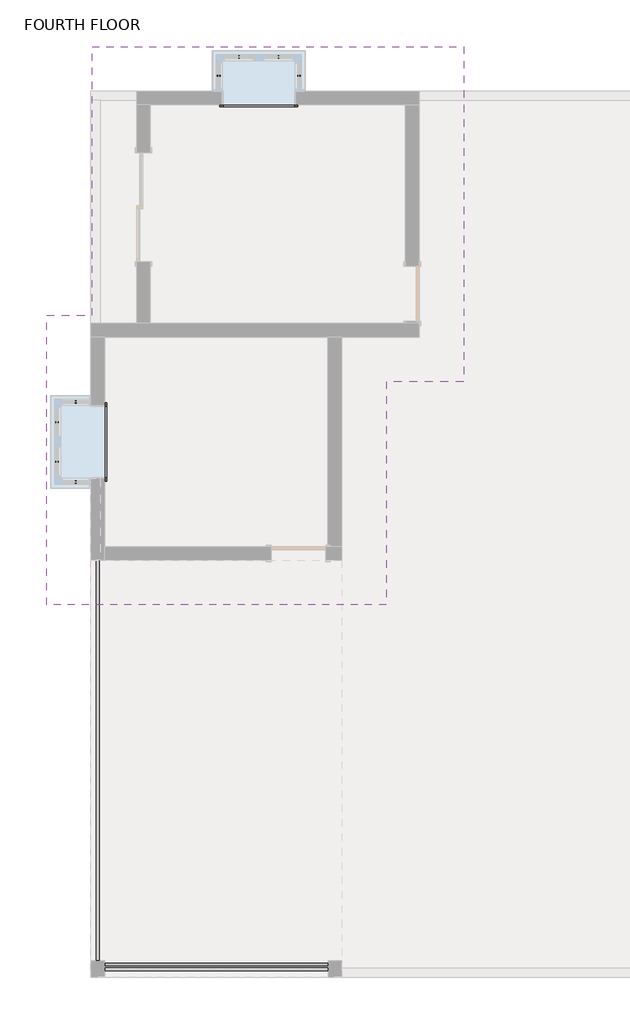
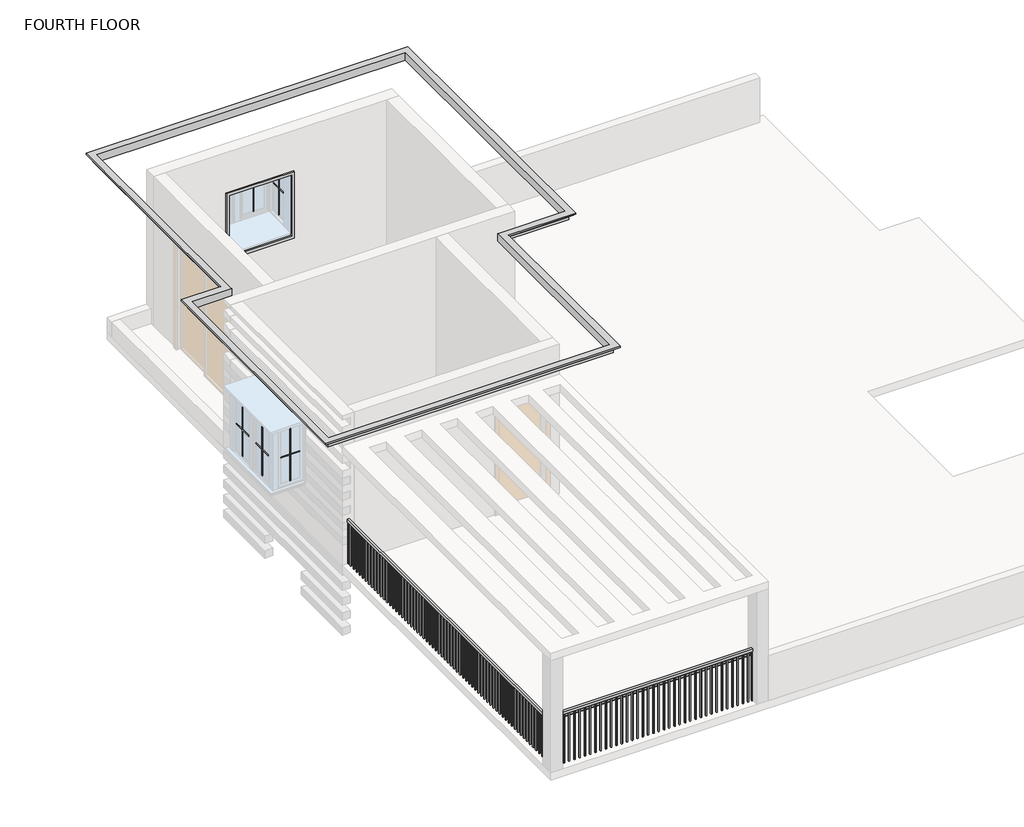
# One storey, part 2 of 2: 11 proxies, 2 railings.
"""IFC4 building model written with IfcOpenShell, lengths in millimetres."""

from ifc_helpers import new_model, si_unit, point, frame, frame_2d, origin, place, context, project, spatial, polyline, circle_curve, trimmed, segment, composite_curve, outline, extrude, transform, mapped, element, save
from components import generic_models_1_generic_models_1_7431621c, muntin_pattern_2x2_muntin_pattern_2x2_4aee108e, muntin_pattern_2x2_muntin_pattern_2x2_f03ab90d, muntin_pattern_2x2_muntin_pattern_2x2_eb08c668, trim_window_interior_flat_picture_frame_ace0ae79

model = new_model("IFC4")

# Units and contexts
model_context = context("Model", 3, world=origin())
ifc_project = project(units=[si_unit("LENGTHUNIT", "METRE", prefix="MILLI")], contexts=[model_context])

# Site, building, storey
site = spatial("IfcSite", under=ifc_project)
building = spatial("IfcBuilding", under=site)
storey = spatial("IfcBuildingStorey", under=building, Name="FOURTH FLOOR", Elevation=12801.6)

# Proxies
placement = place(None, origin())
generic_models_1_generic_models_1_shape = generic_models_1_generic_models_1_7431621c(model_context)
element("IfcBuildingElementProxy", 1, Name="Generic Models 1 : Generic Models 1", ObjectType="Generic Models 1 : Generic Models 1", at=placement, inside=storey, context=model_context, shape_type="MappedRepresentation", body=[
    mapped(generic_models_1_generic_models_1_shape, transform((0.0, 0.0, 0.0), x_axis=(1.0, 0.0, 0.0), y_axis=(0.0, 1.0, 0.0), z_axis=(0.0, 0.0, 1.0))),
])
muntin_pattern_2x2_muntin_pattern_2x2_shape = muntin_pattern_2x2_muntin_pattern_2x2_4aee108e(model_context)
element("IfcBuildingElementProxy", 2, Name="Muntin Pattern_2x2 : Muntin Pattern_2x2", ObjectType="Muntin Pattern_2x2 : Muntin Pattern_2x2", at=placement, inside=storey, context=model_context, shape_type="MappedRepresentation", body=[
    mapped(muntin_pattern_2x2_muntin_pattern_2x2_shape, transform((-4531.8415084, 8637.658346, 13836.65), x_axis=(1.0, 0.0, 0.0), y_axis=(0.0, 1.0, 0.0), z_axis=(0.0, 0.0, 1.0))),
])
element("IfcBuildingElementProxy", 3, Name="Muntin Pattern_2x2 : Muntin Pattern_2x2", ObjectType="Muntin Pattern_2x2 : Muntin Pattern_2x2", at=placement, inside=storey, context=model_context, shape_type="MappedRepresentation", body=[
    mapped(muntin_pattern_2x2_muntin_pattern_2x2_shape, transform((-7576.6665084, 1871.733346, 13836.65), x_axis=(0.0, 1.0, 0.0), y_axis=(-1.0, 0.0, 0.0), z_axis=(0.0, 0.0, 1.0))),
])
muntin_pattern_2x2_muntin_pattern_2x2_2_shape = muntin_pattern_2x2_muntin_pattern_2x2_f03ab90d(model_context)
element("IfcBuildingElementProxy", 4, Name="Muntin Pattern_2x2 : Muntin Pattern_2x2", ObjectType="Muntin Pattern_2x2 : Muntin Pattern_2x2", at=placement, inside=storey, context=model_context, shape_type="MappedRepresentation", body=[
    mapped(muntin_pattern_2x2_muntin_pattern_2x2_2_shape, transform((-4871.5665084, 8323.333346, 13836.65), x_axis=(0.0, -1.0, 0.0), y_axis=(1.0, 0.0, 0.0), z_axis=(0.0, 0.0, 1.0))),
])
element("IfcBuildingElementProxy", 5, Name="Muntin Pattern_2x2 : Muntin Pattern_2x2", ObjectType="Muntin Pattern_2x2 : Muntin Pattern_2x2", at=placement, inside=storey, context=model_context, shape_type="MappedRepresentation", body=[
    mapped(muntin_pattern_2x2_muntin_pattern_2x2_2_shape, transform((-3531.7165084, 8323.333346, 13836.65), x_axis=(0.0, 1.0, 0.0), y_axis=(-1.0, 0.0, 0.0), z_axis=(0.0, 0.0, 1.0))),
])
element("IfcBuildingElementProxy", 6, Name="Muntin Pattern_2x2 : Muntin Pattern_2x2", ObjectType="Muntin Pattern_2x2 : Muntin Pattern_2x2", at=placement, inside=storey, context=model_context, shape_type="MappedRepresentation", body=[
    mapped(muntin_pattern_2x2_muntin_pattern_2x2_2_shape, transform((-7262.3415084, 1532.008346, 13836.65), x_axis=(1.0, 0.0, 0.0), y_axis=(0.0, 1.0, 0.0), z_axis=(0.0, 0.0, 1.0))),
])
element("IfcBuildingElementProxy", 7, Name="Muntin Pattern_2x2 : Muntin Pattern_2x2", ObjectType="Muntin Pattern_2x2 : Muntin Pattern_2x2", at=placement, inside=storey, context=model_context, shape_type="MappedRepresentation", body=[
    mapped(muntin_pattern_2x2_muntin_pattern_2x2_2_shape, transform((-7262.3415084, 2871.858346, 13836.65), x_axis=(-1.0, 0.0, 0.0), y_axis=(0.0, -1.0, 0.0), z_axis=(0.0, 0.0, 1.0))),
])
muntin_pattern_2x2_muntin_pattern_2x2_3_shape = muntin_pattern_2x2_muntin_pattern_2x2_eb08c668(model_context)
element("IfcBuildingElementProxy", 8, Name="Muntin Pattern_2x2 : Muntin Pattern_2x2", ObjectType="Muntin Pattern_2x2 : Muntin Pattern_2x2", at=placement, inside=storey, context=model_context, shape_type="MappedRepresentation", body=[
    mapped(muntin_pattern_2x2_muntin_pattern_2x2_3_shape, transform((-3871.4415084, 8637.658346, 13836.65), x_axis=(-1.0, 0.0, 0.0), y_axis=(0.0, -1.0, 0.0), z_axis=(0.0, 0.0, 1.0))),
])
element("IfcBuildingElementProxy", 9, Name="Muntin Pattern_2x2 : Muntin Pattern_2x2", ObjectType="Muntin Pattern_2x2 : Muntin Pattern_2x2", at=placement, inside=storey, context=model_context, shape_type="MappedRepresentation", body=[
    mapped(muntin_pattern_2x2_muntin_pattern_2x2_3_shape, transform((-7576.6665084, 2532.133346, 13836.65), x_axis=(0.0, -1.0, 0.0), y_axis=(1.0, 0.0, 0.0), z_axis=(0.0, 0.0, 1.0))),
])
trim_window_interior_flat_picture_frame_shape = trim_window_interior_flat_picture_frame_ace0ae79(model_context)
element("IfcBuildingElementProxy", 10, Name="Trim-Window-Interior-Flat : Picture Frame", ObjectType="Trim-Window-Interior-Flat : Picture Frame", at=placement, inside=storey, context=model_context, shape_type="MappedRepresentation", body=[
    mapped(trim_window_interior_flat_picture_frame_shape, transform((-4201.6415084, 7840.733346, 14986.0), x_axis=(1.0, 0.0, 0.0), y_axis=(0.0, 0.0, 1.0), z_axis=(0.0, -1.0, 0.0))),
])
element("IfcBuildingElementProxy", 11, Name="Trim-Window-Interior-Flat : Picture Frame", ObjectType="Trim-Window-Interior-Flat : Picture Frame", at=placement, inside=storey, context=model_context, shape_type="MappedRepresentation", body=[
    mapped(trim_window_interior_flat_picture_frame_shape, transform((-6779.7415084, 2201.933346, 14986.0), x_axis=(0.0, 1.0, 0.0), y_axis=(0.0, 0.0, 1.0), z_axis=(1.0, 0.0, 0.0))),
])

# Railings
element("IfcRailing", 12, ObjectType="Guardrail - Rectangular", at=placement, inside=storey, context=model_context, shape_type="SweptSolid", body=[
    extrude(outline(composite_curve([segment(trimmed(circle_curve(frame_2d((-6535.666654, 13696.95)), 19.05), [point((-6554.716654, 13696.95))], [point((-6516.616654, 13696.95))], False, "CARTESIAN"), True, "CONTINUOUS"), segment(trimmed(circle_curve(frame_2d((-6535.666654, 13696.95)), 19.05), [point((-6516.616654, 13696.95))], [point((-6554.716654, 13696.95))], False, "CARTESIAN"), True, "CONTINUOUS")], self_intersect=False)), frame((-6779.7415084, 0.0, 0.0), z_axis=(1.0, 0.0, 0.0), x_axis=(0.0, 1.0, 0.0)), (0.0, 0.0, 1.0), 3739.3665543),
    extrude(outline(polyline([(-6779.7415084, -6637.266654), (-6779.7415084, -6586.466654), (-3040.3749541, -6586.466654), (-3040.3749541, -6637.266654), (-6779.7415084, -6637.266654)])), frame((0.0, 0.0, 13817.6), z_axis=(0.0, 0.0, 1.0), x_axis=(1.0, 0.0, 0.0)), (0.0, 0.0, 1.0), 50.8),
    extrude(outline(polyline([(-3131.6665084, -6621.391654), (-3131.6665084, -6602.341654), (-3112.6165084, -6602.341654), (-3112.6165084, -6621.391654), (-3131.6665084, -6621.391654)])), frame((0.0, 0.0, 12801.6), z_axis=(0.0, 0.0, 1.0), x_axis=(1.0, 0.0, 0.0)), (0.0, 0.0, 1.0), 1016.0),
    extrude(outline(polyline([(-3233.2665084, -6621.391654), (-3233.2665084, -6602.341654), (-3214.2165084, -6602.341654), (-3214.2165084, -6621.391654), (-3233.2665084, -6621.391654)])), frame((0.0, 0.0, 12801.6), z_axis=(0.0, 0.0, 1.0), x_axis=(1.0, 0.0, 0.0)), (0.0, 0.0, 1.0), 1016.0),
    extrude(outline(polyline([(-3334.8665084, -6621.391654), (-3334.8665084, -6602.341654), (-3315.8165084, -6602.341654), (-3315.8165084, -6621.391654), (-3334.8665084, -6621.391654)])), frame((0.0, 0.0, 12801.6), z_axis=(0.0, 0.0, 1.0), x_axis=(1.0, 0.0, 0.0)), (0.0, 0.0, 1.0), 1016.0),
    extrude(outline(polyline([(-3436.4665084, -6621.391654), (-3436.4665084, -6602.341654), (-3417.4165084, -6602.341654), (-3417.4165084, -6621.391654), (-3436.4665084, -6621.391654)])), frame((0.0, 0.0, 12801.6), z_axis=(0.0, 0.0, 1.0), x_axis=(1.0, 0.0, 0.0)), (0.0, 0.0, 1.0), 1016.0),
    extrude(outline(polyline([(-3538.0665084, -6621.391654), (-3538.0665084, -6602.341654), (-3519.0165084, -6602.341654), (-3519.0165084, -6621.391654), (-3538.0665084, -6621.391654)])), frame((0.0, 0.0, 12801.6), z_axis=(0.0, 0.0, 1.0), x_axis=(1.0, 0.0, 0.0)), (0.0, 0.0, 1.0), 1016.0),
    extrude(outline(polyline([(-3639.6665084, -6621.391654), (-3639.6665084, -6602.341654), (-3620.6165084, -6602.341654), (-3620.6165084, -6621.391654), (-3639.6665084, -6621.391654)])), frame((0.0, 0.0, 12801.6), z_axis=(0.0, 0.0, 1.0), x_axis=(1.0, 0.0, 0.0)), (0.0, 0.0, 1.0), 1016.0),
    extrude(outline(polyline([(-3741.2665084, -6621.391654), (-3741.2665084, -6602.341654), (-3722.2165084, -6602.341654), (-3722.2165084, -6621.391654), (-3741.2665084, -6621.391654)])), frame((0.0, 0.0, 12801.6), z_axis=(0.0, 0.0, 1.0), x_axis=(1.0, 0.0, 0.0)), (0.0, 0.0, 1.0), 1016.0),
    extrude(outline(polyline([(-3842.8665084, -6621.391654), (-3842.8665084, -6602.341654), (-3823.8165084, -6602.341654), (-3823.8165084, -6621.391654), (-3842.8665084, -6621.391654)])), frame((0.0, 0.0, 12801.6), z_axis=(0.0, 0.0, 1.0), x_axis=(1.0, 0.0, 0.0)), (0.0, 0.0, 1.0), 1016.0),
    extrude(outline(polyline([(-3944.4665084, -6621.391654), (-3944.4665084, -6602.341654), (-3925.4165084, -6602.341654), (-3925.4165084, -6621.391654), (-3944.4665084, -6621.391654)])), frame((0.0, 0.0, 12801.6), z_axis=(0.0, 0.0, 1.0), x_axis=(1.0, 0.0, 0.0)), (0.0, 0.0, 1.0), 1016.0),
    extrude(outline(polyline([(-4046.0665084, -6621.391654), (-4046.0665084, -6602.341654), (-4027.0165084, -6602.341654), (-4027.0165084, -6621.391654), (-4046.0665084, -6621.391654)])), frame((0.0, 0.0, 12801.6), z_axis=(0.0, 0.0, 1.0), x_axis=(1.0, 0.0, 0.0)), (0.0, 0.0, 1.0), 1016.0),
    extrude(outline(polyline([(-4147.6665084, -6621.391654), (-4147.6665084, -6602.341654), (-4128.6165084, -6602.341654), (-4128.6165084, -6621.391654), (-4147.6665084, -6621.391654)])), frame((0.0, 0.0, 12801.6), z_axis=(0.0, 0.0, 1.0), x_axis=(1.0, 0.0, 0.0)), (0.0, 0.0, 1.0), 1016.0),
    extrude(outline(polyline([(-4249.2665084, -6621.391654), (-4249.2665084, -6602.341654), (-4230.2165084, -6602.341654), (-4230.2165084, -6621.391654), (-4249.2665084, -6621.391654)])), frame((0.0, 0.0, 12801.6), z_axis=(0.0, 0.0, 1.0), x_axis=(1.0, 0.0, 0.0)), (0.0, 0.0, 1.0), 1016.0),
    extrude(outline(polyline([(-4350.8665084, -6621.391654), (-4350.8665084, -6602.341654), (-4331.8165084, -6602.341654), (-4331.8165084, -6621.391654), (-4350.8665084, -6621.391654)])), frame((0.0, 0.0, 12801.6), z_axis=(0.0, 0.0, 1.0), x_axis=(1.0, 0.0, 0.0)), (0.0, 0.0, 1.0), 1016.0),
    extrude(outline(polyline([(-4452.4665084, -6621.391654), (-4452.4665084, -6602.341654), (-4433.4165084, -6602.341654), (-4433.4165084, -6621.391654), (-4452.4665084, -6621.391654)])), frame((0.0, 0.0, 12801.6), z_axis=(0.0, 0.0, 1.0), x_axis=(1.0, 0.0, 0.0)), (0.0, 0.0, 1.0), 1016.0),
    extrude(outline(polyline([(-4554.0665084, -6621.391654), (-4554.0665084, -6602.341654), (-4535.0165084, -6602.341654), (-4535.0165084, -6621.391654), (-4554.0665084, -6621.391654)])), frame((0.0, 0.0, 12801.6), z_axis=(0.0, 0.0, 1.0), x_axis=(1.0, 0.0, 0.0)), (0.0, 0.0, 1.0), 1016.0),
    extrude(outline(polyline([(-4655.6665084, -6621.391654), (-4655.6665084, -6602.341654), (-4636.6165084, -6602.341654), (-4636.6165084, -6621.391654), (-4655.6665084, -6621.391654)])), frame((0.0, 0.0, 12801.6), z_axis=(0.0, 0.0, 1.0), x_axis=(1.0, 0.0, 0.0)), (0.0, 0.0, 1.0), 1016.0),
    extrude(outline(polyline([(-4757.2665084, -6621.391654), (-4757.2665084, -6602.341654), (-4738.2165084, -6602.341654), (-4738.2165084, -6621.391654), (-4757.2665084, -6621.391654)])), frame((0.0, 0.0, 12801.6), z_axis=(0.0, 0.0, 1.0), x_axis=(1.0, 0.0, 0.0)), (0.0, 0.0, 1.0), 1016.0),
    extrude(outline(polyline([(-4858.8665084, -6621.391654), (-4858.8665084, -6602.341654), (-4839.8165084, -6602.341654), (-4839.8165084, -6621.391654), (-4858.8665084, -6621.391654)])), frame((0.0, 0.0, 12801.6), z_axis=(0.0, 0.0, 1.0), x_axis=(1.0, 0.0, 0.0)), (0.0, 0.0, 1.0), 1016.0),
    extrude(outline(polyline([(-4960.4665084, -6621.391654), (-4960.4665084, -6602.341654), (-4941.4165084, -6602.341654), (-4941.4165084, -6621.391654), (-4960.4665084, -6621.391654)])), frame((0.0, 0.0, 12801.6), z_axis=(0.0, 0.0, 1.0), x_axis=(1.0, 0.0, 0.0)), (0.0, 0.0, 1.0), 1016.0),
    extrude(outline(polyline([(-5062.0665084, -6621.391654), (-5062.0665084, -6602.341654), (-5043.0165084, -6602.341654), (-5043.0165084, -6621.391654), (-5062.0665084, -6621.391654)])), frame((0.0, 0.0, 12801.6), z_axis=(0.0, 0.0, 1.0), x_axis=(1.0, 0.0, 0.0)), (0.0, 0.0, 1.0), 1016.0),
    extrude(outline(polyline([(-5163.6665084, -6621.391654), (-5163.6665084, -6602.341654), (-5144.6165084, -6602.341654), (-5144.6165084, -6621.391654), (-5163.6665084, -6621.391654)])), frame((0.0, 0.0, 12801.6), z_axis=(0.0, 0.0, 1.0), x_axis=(1.0, 0.0, 0.0)), (0.0, 0.0, 1.0), 1016.0),
    extrude(outline(polyline([(-5265.2665084, -6621.391654), (-5265.2665084, -6602.341654), (-5246.2165084, -6602.341654), (-5246.2165084, -6621.391654), (-5265.2665084, -6621.391654)])), frame((0.0, 0.0, 12801.6), z_axis=(0.0, 0.0, 1.0), x_axis=(1.0, 0.0, 0.0)), (0.0, 0.0, 1.0), 1016.0),
    extrude(outline(polyline([(-5366.8665084, -6621.391654), (-5366.8665084, -6602.341654), (-5347.8165084, -6602.341654), (-5347.8165084, -6621.391654), (-5366.8665084, -6621.391654)])), frame((0.0, 0.0, 12801.6), z_axis=(0.0, 0.0, 1.0), x_axis=(1.0, 0.0, 0.0)), (0.0, 0.0, 1.0), 1016.0),
    extrude(outline(polyline([(-5468.4665084, -6621.391654), (-5468.4665084, -6602.341654), (-5449.4165084, -6602.341654), (-5449.4165084, -6621.391654), (-5468.4665084, -6621.391654)])), frame((0.0, 0.0, 12801.6), z_axis=(0.0, 0.0, 1.0), x_axis=(1.0, 0.0, 0.0)), (0.0, 0.0, 1.0), 1016.0),
    extrude(outline(polyline([(-5570.0665084, -6621.391654), (-5570.0665084, -6602.341654), (-5551.0165084, -6602.341654), (-5551.0165084, -6621.391654), (-5570.0665084, -6621.391654)])), frame((0.0, 0.0, 12801.6), z_axis=(0.0, 0.0, 1.0), x_axis=(1.0, 0.0, 0.0)), (0.0, 0.0, 1.0), 1016.0),
    extrude(outline(polyline([(-5671.6665084, -6621.391654), (-5671.6665084, -6602.341654), (-5652.6165084, -6602.341654), (-5652.6165084, -6621.391654), (-5671.6665084, -6621.391654)])), frame((0.0, 0.0, 12801.6), z_axis=(0.0, 0.0, 1.0), x_axis=(1.0, 0.0, 0.0)), (0.0, 0.0, 1.0), 1016.0),
    extrude(outline(polyline([(-5773.2665084, -6621.391654), (-5773.2665084, -6602.341654), (-5754.2165084, -6602.341654), (-5754.2165084, -6621.391654), (-5773.2665084, -6621.391654)])), frame((0.0, 0.0, 12801.6), z_axis=(0.0, 0.0, 1.0), x_axis=(1.0, 0.0, 0.0)), (0.0, 0.0, 1.0), 1016.0),
    extrude(outline(polyline([(-5874.8665084, -6621.391654), (-5874.8665084, -6602.341654), (-5855.8165084, -6602.341654), (-5855.8165084, -6621.391654), (-5874.8665084, -6621.391654)])), frame((0.0, 0.0, 12801.6), z_axis=(0.0, 0.0, 1.0), x_axis=(1.0, 0.0, 0.0)), (0.0, 0.0, 1.0), 1016.0),
    extrude(outline(polyline([(-5976.4665084, -6621.391654), (-5976.4665084, -6602.341654), (-5957.4165084, -6602.341654), (-5957.4165084, -6621.391654), (-5976.4665084, -6621.391654)])), frame((0.0, 0.0, 12801.6), z_axis=(0.0, 0.0, 1.0), x_axis=(1.0, 0.0, 0.0)), (0.0, 0.0, 1.0), 1016.0),
    extrude(outline(polyline([(-6078.0665084, -6621.391654), (-6078.0665084, -6602.341654), (-6059.0165084, -6602.341654), (-6059.0165084, -6621.391654), (-6078.0665084, -6621.391654)])), frame((0.0, 0.0, 12801.6), z_axis=(0.0, 0.0, 1.0), x_axis=(1.0, 0.0, 0.0)), (0.0, 0.0, 1.0), 1016.0),
    extrude(outline(polyline([(-6179.6665084, -6621.391654), (-6179.6665084, -6602.341654), (-6160.6165084, -6602.341654), (-6160.6165084, -6621.391654), (-6179.6665084, -6621.391654)])), frame((0.0, 0.0, 12801.6), z_axis=(0.0, 0.0, 1.0), x_axis=(1.0, 0.0, 0.0)), (0.0, 0.0, 1.0), 1016.0),
    extrude(outline(polyline([(-6281.2665084, -6621.391654), (-6281.2665084, -6602.341654), (-6262.2165084, -6602.341654), (-6262.2165084, -6621.391654), (-6281.2665084, -6621.391654)])), frame((0.0, 0.0, 12801.6), z_axis=(0.0, 0.0, 1.0), x_axis=(1.0, 0.0, 0.0)), (0.0, 0.0, 1.0), 1016.0),
    extrude(outline(polyline([(-6382.8665084, -6621.391654), (-6382.8665084, -6602.341654), (-6363.8165084, -6602.341654), (-6363.8165084, -6621.391654), (-6382.8665084, -6621.391654)])), frame((0.0, 0.0, 12801.6), z_axis=(0.0, 0.0, 1.0), x_axis=(1.0, 0.0, 0.0)), (0.0, 0.0, 1.0), 1016.0),
    extrude(outline(polyline([(-6484.4665084, -6621.391654), (-6484.4665084, -6602.341654), (-6465.4165084, -6602.341654), (-6465.4165084, -6621.391654), (-6484.4665084, -6621.391654)])), frame((0.0, 0.0, 12801.6), z_axis=(0.0, 0.0, 1.0), x_axis=(1.0, 0.0, 0.0)), (0.0, 0.0, 1.0), 1016.0),
    extrude(outline(polyline([(-6586.0665084, -6621.391654), (-6586.0665084, -6602.341654), (-6567.0165084, -6602.341654), (-6567.0165084, -6621.391654), (-6586.0665084, -6621.391654)])), frame((0.0, 0.0, 12801.6), z_axis=(0.0, 0.0, 1.0), x_axis=(1.0, 0.0, 0.0)), (0.0, 0.0, 1.0), 1016.0),
    extrude(outline(polyline([(-6687.6665084, -6621.391654), (-6687.6665084, -6602.341654), (-6668.6165084, -6602.341654), (-6668.6165084, -6621.391654), (-6687.6665084, -6621.391654)])), frame((0.0, 0.0, 12801.6), z_axis=(0.0, 0.0, 1.0), x_axis=(1.0, 0.0, 0.0)), (0.0, 0.0, 1.0), 1016.0),
    extrude(outline(polyline([(-3059.4249541, -6621.391654), (-3059.4249541, -6602.341654), (-3040.3749541, -6602.341654), (-3040.3749541, -6621.391654), (-3059.4249541, -6621.391654)])), frame((0.0, 0.0, 12801.6), z_axis=(0.0, 0.0, 1.0), x_axis=(1.0, 0.0, 0.0)), (0.0, 0.0, 1.0), 1016.0),
    extrude(outline(polyline([(-6779.7415084, -6621.391654), (-6779.7415084, -6602.341654), (-6760.6915084, -6602.341654), (-6760.6915084, -6621.391654), (-6779.7415084, -6621.391654)])), frame((0.0, 0.0, 12801.6), z_axis=(0.0, 0.0, 1.0), x_axis=(1.0, 0.0, 0.0)), (0.0, 0.0, 1.0), 1016.0),
])
element("IfcRailing", 13, ObjectType="Handrail - Rectangular", at=placement, inside=storey, context=model_context, shape_type="SweptSolid", body=[
    extrude(outline(polyline([(-6868.6415084, -6472.166654), (-6919.4415084, -6472.166654), (-6919.4415084, 220.733346), (-6868.6415084, 220.733346), (-6868.6415084, -6472.166654)])), frame((0.0, 0.0, 13665.2), z_axis=(0.0, 0.0, 1.0), x_axis=(1.0, 0.0, 0.0)), (0.0, 0.0, 1.0), 50.8),
    extrude(outline(polyline([(-6884.5165084, 122.308346), (-6903.5665084, 122.308346), (-6903.5665084, 141.358346), (-6884.5165084, 141.358346), (-6884.5165084, 122.308346)])), frame((0.0, 0.0, 12801.6), z_axis=(0.0, 0.0, 1.0), x_axis=(1.0, 0.0, 0.0)), (0.0, 0.0, 1.0), 863.6),
    extrude(outline(polyline([(-6884.5165084, 20.708346), (-6903.5665084, 20.708346), (-6903.5665084, 39.758346), (-6884.5165084, 39.758346), (-6884.5165084, 20.708346)])), frame((0.0, 0.0, 12801.6), z_axis=(0.0, 0.0, 1.0), x_axis=(1.0, 0.0, 0.0)), (0.0, 0.0, 1.0), 863.6),
    extrude(outline(polyline([(-6884.5165084, -80.891654), (-6903.5665084, -80.891654), (-6903.5665084, -61.841654), (-6884.5165084, -61.841654), (-6884.5165084, -80.891654)])), frame((0.0, 0.0, 12801.6), z_axis=(0.0, 0.0, 1.0), x_axis=(1.0, 0.0, 0.0)), (0.0, 0.0, 1.0), 863.6),
    extrude(outline(polyline([(-6884.5165084, -182.491654), (-6903.5665084, -182.491654), (-6903.5665084, -163.441654), (-6884.5165084, -163.441654), (-6884.5165084, -182.491654)])), frame((0.0, 0.0, 12801.6), z_axis=(0.0, 0.0, 1.0), x_axis=(1.0, 0.0, 0.0)), (0.0, 0.0, 1.0), 863.6),
    extrude(outline(polyline([(-6884.5165084, -284.091654), (-6903.5665084, -284.091654), (-6903.5665084, -265.041654), (-6884.5165084, -265.041654), (-6884.5165084, -284.091654)])), frame((0.0, 0.0, 12801.6), z_axis=(0.0, 0.0, 1.0), x_axis=(1.0, 0.0, 0.0)), (0.0, 0.0, 1.0), 863.6),
    extrude(outline(polyline([(-6884.5165084, -385.691654), (-6903.5665084, -385.691654), (-6903.5665084, -366.641654), (-6884.5165084, -366.641654), (-6884.5165084, -385.691654)])), frame((0.0, 0.0, 12801.6), z_axis=(0.0, 0.0, 1.0), x_axis=(1.0, 0.0, 0.0)), (0.0, 0.0, 1.0), 863.6),
    extrude(outline(polyline([(-6884.5165084, -487.291654), (-6903.5665084, -487.291654), (-6903.5665084, -468.241654), (-6884.5165084, -468.241654), (-6884.5165084, -487.291654)])), frame((0.0, 0.0, 12801.6), z_axis=(0.0, 0.0, 1.0), x_axis=(1.0, 0.0, 0.0)), (0.0, 0.0, 1.0), 863.6),
    extrude(outline(polyline([(-6884.5165084, -588.891654), (-6903.5665084, -588.891654), (-6903.5665084, -569.841654), (-6884.5165084, -569.841654), (-6884.5165084, -588.891654)])), frame((0.0, 0.0, 12801.6), z_axis=(0.0, 0.0, 1.0), x_axis=(1.0, 0.0, 0.0)), (0.0, 0.0, 1.0), 863.6),
    extrude(outline(polyline([(-6884.5165084, -690.491654), (-6903.5665084, -690.491654), (-6903.5665084, -671.441654), (-6884.5165084, -671.441654), (-6884.5165084, -690.491654)])), frame((0.0, 0.0, 12801.6), z_axis=(0.0, 0.0, 1.0), x_axis=(1.0, 0.0, 0.0)), (0.0, 0.0, 1.0), 863.6),
    extrude(outline(polyline([(-6884.5165084, -792.091654), (-6903.5665084, -792.091654), (-6903.5665084, -773.041654), (-6884.5165084, -773.041654), (-6884.5165084, -792.091654)])), frame((0.0, 0.0, 12801.6), z_axis=(0.0, 0.0, 1.0), x_axis=(1.0, 0.0, 0.0)), (0.0, 0.0, 1.0), 863.6),
    extrude(outline(polyline([(-6884.5165084, -893.691654), (-6903.5665084, -893.691654), (-6903.5665084, -874.641654), (-6884.5165084, -874.641654), (-6884.5165084, -893.691654)])), frame((0.0, 0.0, 12801.6), z_axis=(0.0, 0.0, 1.0), x_axis=(1.0, 0.0, 0.0)), (0.0, 0.0, 1.0), 863.6),
    extrude(outline(polyline([(-6884.5165084, -995.291654), (-6903.5665084, -995.291654), (-6903.5665084, -976.241654), (-6884.5165084, -976.241654), (-6884.5165084, -995.291654)])), frame((0.0, 0.0, 12801.6), z_axis=(0.0, 0.0, 1.0), x_axis=(1.0, 0.0, 0.0)), (0.0, 0.0, 1.0), 863.6),
    extrude(outline(polyline([(-6884.5165084, -1096.891654), (-6903.5665084, -1096.891654), (-6903.5665084, -1077.841654), (-6884.5165084, -1077.841654), (-6884.5165084, -1096.891654)])), frame((0.0, 0.0, 12801.6), z_axis=(0.0, 0.0, 1.0), x_axis=(1.0, 0.0, 0.0)), (0.0, 0.0, 1.0), 863.6),
    extrude(outline(polyline([(-6884.5165084, -1198.491654), (-6903.5665084, -1198.491654), (-6903.5665084, -1179.441654), (-6884.5165084, -1179.441654), (-6884.5165084, -1198.491654)])), frame((0.0, 0.0, 12801.6), z_axis=(0.0, 0.0, 1.0), x_axis=(1.0, 0.0, 0.0)), (0.0, 0.0, 1.0), 863.6),
    extrude(outline(polyline([(-6884.5165084, -1300.091654), (-6903.5665084, -1300.091654), (-6903.5665084, -1281.041654), (-6884.5165084, -1281.041654), (-6884.5165084, -1300.091654)])), frame((0.0, 0.0, 12801.6), z_axis=(0.0, 0.0, 1.0), x_axis=(1.0, 0.0, 0.0)), (0.0, 0.0, 1.0), 863.6),
    extrude(outline(polyline([(-6884.5165084, -1401.691654), (-6903.5665084, -1401.691654), (-6903.5665084, -1382.641654), (-6884.5165084, -1382.641654), (-6884.5165084, -1401.691654)])), frame((0.0, 0.0, 12801.6), z_axis=(0.0, 0.0, 1.0), x_axis=(1.0, 0.0, 0.0)), (0.0, 0.0, 1.0), 863.6),
    extrude(outline(polyline([(-6884.5165084, -1503.291654), (-6903.5665084, -1503.291654), (-6903.5665084, -1484.241654), (-6884.5165084, -1484.241654), (-6884.5165084, -1503.291654)])), frame((0.0, 0.0, 12801.6), z_axis=(0.0, 0.0, 1.0), x_axis=(1.0, 0.0, 0.0)), (0.0, 0.0, 1.0), 863.6),
    extrude(outline(polyline([(-6884.5165084, -1604.891654), (-6903.5665084, -1604.891654), (-6903.5665084, -1585.841654), (-6884.5165084, -1585.841654), (-6884.5165084, -1604.891654)])), frame((0.0, 0.0, 12801.6), z_axis=(0.0, 0.0, 1.0), x_axis=(1.0, 0.0, 0.0)), (0.0, 0.0, 1.0), 863.6),
    extrude(outline(polyline([(-6884.5165084, -1706.491654), (-6903.5665084, -1706.491654), (-6903.5665084, -1687.441654), (-6884.5165084, -1687.441654), (-6884.5165084, -1706.491654)])), frame((0.0, 0.0, 12801.6), z_axis=(0.0, 0.0, 1.0), x_axis=(1.0, 0.0, 0.0)), (0.0, 0.0, 1.0), 863.6),
    extrude(outline(polyline([(-6884.5165084, -1808.091654), (-6903.5665084, -1808.091654), (-6903.5665084, -1789.041654), (-6884.5165084, -1789.041654), (-6884.5165084, -1808.091654)])), frame((0.0, 0.0, 12801.6), z_axis=(0.0, 0.0, 1.0), x_axis=(1.0, 0.0, 0.0)), (0.0, 0.0, 1.0), 863.6),
    extrude(outline(polyline([(-6884.5165084, -1909.691654), (-6903.5665084, -1909.691654), (-6903.5665084, -1890.641654), (-6884.5165084, -1890.641654), (-6884.5165084, -1909.691654)])), frame((0.0, 0.0, 12801.6), z_axis=(0.0, 0.0, 1.0), x_axis=(1.0, 0.0, 0.0)), (0.0, 0.0, 1.0), 863.6),
    extrude(outline(polyline([(-6884.5165084, -2011.291654), (-6903.5665084, -2011.291654), (-6903.5665084, -1992.241654), (-6884.5165084, -1992.241654), (-6884.5165084, -2011.291654)])), frame((0.0, 0.0, 12801.6), z_axis=(0.0, 0.0, 1.0), x_axis=(1.0, 0.0, 0.0)), (0.0, 0.0, 1.0), 863.6),
    extrude(outline(polyline([(-6884.5165084, -2112.891654), (-6903.5665084, -2112.891654), (-6903.5665084, -2093.841654), (-6884.5165084, -2093.841654), (-6884.5165084, -2112.891654)])), frame((0.0, 0.0, 12801.6), z_axis=(0.0, 0.0, 1.0), x_axis=(1.0, 0.0, 0.0)), (0.0, 0.0, 1.0), 863.6),
    extrude(outline(polyline([(-6884.5165084, -2214.491654), (-6903.5665084, -2214.491654), (-6903.5665084, -2195.441654), (-6884.5165084, -2195.441654), (-6884.5165084, -2214.491654)])), frame((0.0, 0.0, 12801.6), z_axis=(0.0, 0.0, 1.0), x_axis=(1.0, 0.0, 0.0)), (0.0, 0.0, 1.0), 863.6),
    extrude(outline(polyline([(-6884.5165084, -2316.091654), (-6903.5665084, -2316.091654), (-6903.5665084, -2297.041654), (-6884.5165084, -2297.041654), (-6884.5165084, -2316.091654)])), frame((0.0, 0.0, 12801.6), z_axis=(0.0, 0.0, 1.0), x_axis=(1.0, 0.0, 0.0)), (0.0, 0.0, 1.0), 863.6),
    extrude(outline(polyline([(-6884.5165084, -2417.691654), (-6903.5665084, -2417.691654), (-6903.5665084, -2398.641654), (-6884.5165084, -2398.641654), (-6884.5165084, -2417.691654)])), frame((0.0, 0.0, 12801.6), z_axis=(0.0, 0.0, 1.0), x_axis=(1.0, 0.0, 0.0)), (0.0, 0.0, 1.0), 863.6),
    extrude(outline(polyline([(-6884.5165084, -2519.291654), (-6903.5665084, -2519.291654), (-6903.5665084, -2500.241654), (-6884.5165084, -2500.241654), (-6884.5165084, -2519.291654)])), frame((0.0, 0.0, 12801.6), z_axis=(0.0, 0.0, 1.0), x_axis=(1.0, 0.0, 0.0)), (0.0, 0.0, 1.0), 863.6),
    extrude(outline(polyline([(-6884.5165084, -2620.891654), (-6903.5665084, -2620.891654), (-6903.5665084, -2601.841654), (-6884.5165084, -2601.841654), (-6884.5165084, -2620.891654)])), frame((0.0, 0.0, 12801.6), z_axis=(0.0, 0.0, 1.0), x_axis=(1.0, 0.0, 0.0)), (0.0, 0.0, 1.0), 863.6),
    extrude(outline(polyline([(-6884.5165084, -2722.491654), (-6903.5665084, -2722.491654), (-6903.5665084, -2703.441654), (-6884.5165084, -2703.441654), (-6884.5165084, -2722.491654)])), frame((0.0, 0.0, 12801.6), z_axis=(0.0, 0.0, 1.0), x_axis=(1.0, 0.0, 0.0)), (0.0, 0.0, 1.0), 863.6),
    extrude(outline(polyline([(-6884.5165084, -2824.091654), (-6903.5665084, -2824.091654), (-6903.5665084, -2805.041654), (-6884.5165084, -2805.041654), (-6884.5165084, -2824.091654)])), frame((0.0, 0.0, 12801.6), z_axis=(0.0, 0.0, 1.0), x_axis=(1.0, 0.0, 0.0)), (0.0, 0.0, 1.0), 863.6),
    extrude(outline(polyline([(-6884.5165084, -2925.691654), (-6903.5665084, -2925.691654), (-6903.5665084, -2906.641654), (-6884.5165084, -2906.641654), (-6884.5165084, -2925.691654)])), frame((0.0, 0.0, 12801.6), z_axis=(0.0, 0.0, 1.0), x_axis=(1.0, 0.0, 0.0)), (0.0, 0.0, 1.0), 863.6),
    extrude(outline(polyline([(-6884.5165084, -3027.291654), (-6903.5665084, -3027.291654), (-6903.5665084, -3008.241654), (-6884.5165084, -3008.241654), (-6884.5165084, -3027.291654)])), frame((0.0, 0.0, 12801.6), z_axis=(0.0, 0.0, 1.0), x_axis=(1.0, 0.0, 0.0)), (0.0, 0.0, 1.0), 863.6),
    extrude(outline(polyline([(-6884.5165084, -3128.891654), (-6903.5665084, -3128.891654), (-6903.5665084, -3109.841654), (-6884.5165084, -3109.841654), (-6884.5165084, -3128.891654)])), frame((0.0, 0.0, 12801.6), z_axis=(0.0, 0.0, 1.0), x_axis=(1.0, 0.0, 0.0)), (0.0, 0.0, 1.0), 863.6),
    extrude(outline(polyline([(-6884.5165084, -3230.491654), (-6903.5665084, -3230.491654), (-6903.5665084, -3211.441654), (-6884.5165084, -3211.441654), (-6884.5165084, -3230.491654)])), frame((0.0, 0.0, 12801.6), z_axis=(0.0, 0.0, 1.0), x_axis=(1.0, 0.0, 0.0)), (0.0, 0.0, 1.0), 863.6),
    extrude(outline(polyline([(-6884.5165084, -3332.091654), (-6903.5665084, -3332.091654), (-6903.5665084, -3313.041654), (-6884.5165084, -3313.041654), (-6884.5165084, -3332.091654)])), frame((0.0, 0.0, 12801.6), z_axis=(0.0, 0.0, 1.0), x_axis=(1.0, 0.0, 0.0)), (0.0, 0.0, 1.0), 863.6),
    extrude(outline(polyline([(-6884.5165084, -3433.691654), (-6903.5665084, -3433.691654), (-6903.5665084, -3414.641654), (-6884.5165084, -3414.641654), (-6884.5165084, -3433.691654)])), frame((0.0, 0.0, 12801.6), z_axis=(0.0, 0.0, 1.0), x_axis=(1.0, 0.0, 0.0)), (0.0, 0.0, 1.0), 863.6),
    extrude(outline(polyline([(-6884.5165084, -3535.291654), (-6903.5665084, -3535.291654), (-6903.5665084, -3516.241654), (-6884.5165084, -3516.241654), (-6884.5165084, -3535.291654)])), frame((0.0, 0.0, 12801.6), z_axis=(0.0, 0.0, 1.0), x_axis=(1.0, 0.0, 0.0)), (0.0, 0.0, 1.0), 863.6),
    extrude(outline(polyline([(-6884.5165084, -3636.891654), (-6903.5665084, -3636.891654), (-6903.5665084, -3617.841654), (-6884.5165084, -3617.841654), (-6884.5165084, -3636.891654)])), frame((0.0, 0.0, 12801.6), z_axis=(0.0, 0.0, 1.0), x_axis=(1.0, 0.0, 0.0)), (0.0, 0.0, 1.0), 863.6),
    extrude(outline(polyline([(-6884.5165084, -3738.491654), (-6903.5665084, -3738.491654), (-6903.5665084, -3719.441654), (-6884.5165084, -3719.441654), (-6884.5165084, -3738.491654)])), frame((0.0, 0.0, 12801.6), z_axis=(0.0, 0.0, 1.0), x_axis=(1.0, 0.0, 0.0)), (0.0, 0.0, 1.0), 863.6),
    extrude(outline(polyline([(-6884.5165084, -3840.091654), (-6903.5665084, -3840.091654), (-6903.5665084, -3821.041654), (-6884.5165084, -3821.041654), (-6884.5165084, -3840.091654)])), frame((0.0, 0.0, 12801.6), z_axis=(0.0, 0.0, 1.0), x_axis=(1.0, 0.0, 0.0)), (0.0, 0.0, 1.0), 863.6),
    extrude(outline(polyline([(-6884.5165084, -3941.691654), (-6903.5665084, -3941.691654), (-6903.5665084, -3922.641654), (-6884.5165084, -3922.641654), (-6884.5165084, -3941.691654)])), frame((0.0, 0.0, 12801.6), z_axis=(0.0, 0.0, 1.0), x_axis=(1.0, 0.0, 0.0)), (0.0, 0.0, 1.0), 863.6),
    extrude(outline(polyline([(-6884.5165084, -4043.291654), (-6903.5665084, -4043.291654), (-6903.5665084, -4024.241654), (-6884.5165084, -4024.241654), (-6884.5165084, -4043.291654)])), frame((0.0, 0.0, 12801.6), z_axis=(0.0, 0.0, 1.0), x_axis=(1.0, 0.0, 0.0)), (0.0, 0.0, 1.0), 863.6),
    extrude(outline(polyline([(-6884.5165084, -4144.891654), (-6903.5665084, -4144.891654), (-6903.5665084, -4125.841654), (-6884.5165084, -4125.841654), (-6884.5165084, -4144.891654)])), frame((0.0, 0.0, 12801.6), z_axis=(0.0, 0.0, 1.0), x_axis=(1.0, 0.0, 0.0)), (0.0, 0.0, 1.0), 863.6),
    extrude(outline(polyline([(-6884.5165084, -4246.491654), (-6903.5665084, -4246.491654), (-6903.5665084, -4227.441654), (-6884.5165084, -4227.441654), (-6884.5165084, -4246.491654)])), frame((0.0, 0.0, 12801.6), z_axis=(0.0, 0.0, 1.0), x_axis=(1.0, 0.0, 0.0)), (0.0, 0.0, 1.0), 863.6),
    extrude(outline(polyline([(-6884.5165084, -4348.091654), (-6903.5665084, -4348.091654), (-6903.5665084, -4329.041654), (-6884.5165084, -4329.041654), (-6884.5165084, -4348.091654)])), frame((0.0, 0.0, 12801.6), z_axis=(0.0, 0.0, 1.0), x_axis=(1.0, 0.0, 0.0)), (0.0, 0.0, 1.0), 863.6),
    extrude(outline(polyline([(-6884.5165084, -4449.691654), (-6903.5665084, -4449.691654), (-6903.5665084, -4430.641654), (-6884.5165084, -4430.641654), (-6884.5165084, -4449.691654)])), frame((0.0, 0.0, 12801.6), z_axis=(0.0, 0.0, 1.0), x_axis=(1.0, 0.0, 0.0)), (0.0, 0.0, 1.0), 863.6),
    extrude(outline(polyline([(-6884.5165084, -4551.291654), (-6903.5665084, -4551.291654), (-6903.5665084, -4532.241654), (-6884.5165084, -4532.241654), (-6884.5165084, -4551.291654)])), frame((0.0, 0.0, 12801.6), z_axis=(0.0, 0.0, 1.0), x_axis=(1.0, 0.0, 0.0)), (0.0, 0.0, 1.0), 863.6),
    extrude(outline(polyline([(-6884.5165084, -4652.891654), (-6903.5665084, -4652.891654), (-6903.5665084, -4633.841654), (-6884.5165084, -4633.841654), (-6884.5165084, -4652.891654)])), frame((0.0, 0.0, 12801.6), z_axis=(0.0, 0.0, 1.0), x_axis=(1.0, 0.0, 0.0)), (0.0, 0.0, 1.0), 863.6),
    extrude(outline(polyline([(-6884.5165084, -4754.491654), (-6903.5665084, -4754.491654), (-6903.5665084, -4735.441654), (-6884.5165084, -4735.441654), (-6884.5165084, -4754.491654)])), frame((0.0, 0.0, 12801.6), z_axis=(0.0, 0.0, 1.0), x_axis=(1.0, 0.0, 0.0)), (0.0, 0.0, 1.0), 863.6),
    extrude(outline(polyline([(-6884.5165084, -4856.091654), (-6903.5665084, -4856.091654), (-6903.5665084, -4837.041654), (-6884.5165084, -4837.041654), (-6884.5165084, -4856.091654)])), frame((0.0, 0.0, 12801.6), z_axis=(0.0, 0.0, 1.0), x_axis=(1.0, 0.0, 0.0)), (0.0, 0.0, 1.0), 863.6),
    extrude(outline(polyline([(-6884.5165084, -4957.691654), (-6903.5665084, -4957.691654), (-6903.5665084, -4938.641654), (-6884.5165084, -4938.641654), (-6884.5165084, -4957.691654)])), frame((0.0, 0.0, 12801.6), z_axis=(0.0, 0.0, 1.0), x_axis=(1.0, 0.0, 0.0)), (0.0, 0.0, 1.0), 863.6),
    extrude(outline(polyline([(-6884.5165084, -5059.291654), (-6903.5665084, -5059.291654), (-6903.5665084, -5040.241654), (-6884.5165084, -5040.241654), (-6884.5165084, -5059.291654)])), frame((0.0, 0.0, 12801.6), z_axis=(0.0, 0.0, 1.0), x_axis=(1.0, 0.0, 0.0)), (0.0, 0.0, 1.0), 863.6),
    extrude(outline(polyline([(-6884.5165084, -5160.891654), (-6903.5665084, -5160.891654), (-6903.5665084, -5141.841654), (-6884.5165084, -5141.841654), (-6884.5165084, -5160.891654)])), frame((0.0, 0.0, 12801.6), z_axis=(0.0, 0.0, 1.0), x_axis=(1.0, 0.0, 0.0)), (0.0, 0.0, 1.0), 863.6),
    extrude(outline(polyline([(-6884.5165084, -5262.491654), (-6903.5665084, -5262.491654), (-6903.5665084, -5243.441654), (-6884.5165084, -5243.441654), (-6884.5165084, -5262.491654)])), frame((0.0, 0.0, 12801.6), z_axis=(0.0, 0.0, 1.0), x_axis=(1.0, 0.0, 0.0)), (0.0, 0.0, 1.0), 863.6),
    extrude(outline(polyline([(-6884.5165084, -5364.091654), (-6903.5665084, -5364.091654), (-6903.5665084, -5345.041654), (-6884.5165084, -5345.041654), (-6884.5165084, -5364.091654)])), frame((0.0, 0.0, 12801.6), z_axis=(0.0, 0.0, 1.0), x_axis=(1.0, 0.0, 0.0)), (0.0, 0.0, 1.0), 863.6),
    extrude(outline(polyline([(-6884.5165084, -5465.691654), (-6903.5665084, -5465.691654), (-6903.5665084, -5446.641654), (-6884.5165084, -5446.641654), (-6884.5165084, -5465.691654)])), frame((0.0, 0.0, 12801.6), z_axis=(0.0, 0.0, 1.0), x_axis=(1.0, 0.0, 0.0)), (0.0, 0.0, 1.0), 863.6),
    extrude(outline(polyline([(-6884.5165084, -5567.291654), (-6903.5665084, -5567.291654), (-6903.5665084, -5548.241654), (-6884.5165084, -5548.241654), (-6884.5165084, -5567.291654)])), frame((0.0, 0.0, 12801.6), z_axis=(0.0, 0.0, 1.0), x_axis=(1.0, 0.0, 0.0)), (0.0, 0.0, 1.0), 863.6),
    extrude(outline(polyline([(-6884.5165084, -5668.891654), (-6903.5665084, -5668.891654), (-6903.5665084, -5649.841654), (-6884.5165084, -5649.841654), (-6884.5165084, -5668.891654)])), frame((0.0, 0.0, 12801.6), z_axis=(0.0, 0.0, 1.0), x_axis=(1.0, 0.0, 0.0)), (0.0, 0.0, 1.0), 863.6),
    extrude(outline(polyline([(-6884.5165084, -5770.491654), (-6903.5665084, -5770.491654), (-6903.5665084, -5751.441654), (-6884.5165084, -5751.441654), (-6884.5165084, -5770.491654)])), frame((0.0, 0.0, 12801.6), z_axis=(0.0, 0.0, 1.0), x_axis=(1.0, 0.0, 0.0)), (0.0, 0.0, 1.0), 863.6),
    extrude(outline(polyline([(-6884.5165084, -5872.091654), (-6903.5665084, -5872.091654), (-6903.5665084, -5853.041654), (-6884.5165084, -5853.041654), (-6884.5165084, -5872.091654)])), frame((0.0, 0.0, 12801.6), z_axis=(0.0, 0.0, 1.0), x_axis=(1.0, 0.0, 0.0)), (0.0, 0.0, 1.0), 863.6),
    extrude(outline(polyline([(-6884.5165084, -5973.691654), (-6903.5665084, -5973.691654), (-6903.5665084, -5954.641654), (-6884.5165084, -5954.641654), (-6884.5165084, -5973.691654)])), frame((0.0, 0.0, 12801.6), z_axis=(0.0, 0.0, 1.0), x_axis=(1.0, 0.0, 0.0)), (0.0, 0.0, 1.0), 863.6),
    extrude(outline(polyline([(-6884.5165084, -6075.291654), (-6903.5665084, -6075.291654), (-6903.5665084, -6056.241654), (-6884.5165084, -6056.241654), (-6884.5165084, -6075.291654)])), frame((0.0, 0.0, 12801.6), z_axis=(0.0, 0.0, 1.0), x_axis=(1.0, 0.0, 0.0)), (0.0, 0.0, 1.0), 863.6),
    extrude(outline(polyline([(-6884.5165084, -6176.891654), (-6903.5665084, -6176.891654), (-6903.5665084, -6157.841654), (-6884.5165084, -6157.841654), (-6884.5165084, -6176.891654)])), frame((0.0, 0.0, 12801.6), z_axis=(0.0, 0.0, 1.0), x_axis=(1.0, 0.0, 0.0)), (0.0, 0.0, 1.0), 863.6),
    extrude(outline(polyline([(-6884.5165084, -6278.491654), (-6903.5665084, -6278.491654), (-6903.5665084, -6259.441654), (-6884.5165084, -6259.441654), (-6884.5165084, -6278.491654)])), frame((0.0, 0.0, 12801.6), z_axis=(0.0, 0.0, 1.0), x_axis=(1.0, 0.0, 0.0)), (0.0, 0.0, 1.0), 863.6),
    extrude(outline(polyline([(-6884.5165084, -6380.091654), (-6903.5665084, -6380.091654), (-6903.5665084, -6361.041654), (-6884.5165084, -6361.041654), (-6884.5165084, -6380.091654)])), frame((0.0, 0.0, 12801.6), z_axis=(0.0, 0.0, 1.0), x_axis=(1.0, 0.0, 0.0)), (0.0, 0.0, 1.0), 863.6),
    extrude(outline(polyline([(-6884.5165084, 201.683346), (-6903.5665084, 201.683346), (-6903.5665084, 220.733346), (-6884.5165084, 220.733346), (-6884.5165084, 201.683346)])), frame((0.0, 0.0, 12801.6), z_axis=(0.0, 0.0, 1.0), x_axis=(1.0, 0.0, 0.0)), (0.0, 0.0, 1.0), 863.6),
    extrude(outline(polyline([(-6884.5165084, -6472.166654), (-6903.5665084, -6472.166654), (-6903.5665084, -6453.116654), (-6884.5165084, -6453.116654), (-6884.5165084, -6472.166654)])), frame((0.0, 0.0, 12801.6), z_axis=(0.0, 0.0, 1.0), x_axis=(1.0, 0.0, 0.0)), (0.0, 0.0, 1.0), 863.6),
])

save(model, "model.ifc")

# Revit data of these elements
# Type "Muntin Pattern_2x2 : Muntin Pattern_2x2"
#   Width [instance default] = 4' - 0"
#   Thickness = 0' - 0 1/2"
#   Height [instance default] = 4' - 0"
#   Distance = 0' - 0 3/4"
#   Interior Material [instance default] = none
#   Exterior Material [instance default] = none
#   Default Elevation = 0
# Type "Trim-Window-Interior-Flat : Picture Frame"
#   Trim Thickness_Picture Frame = 0' - 1 1/4"
#   Trim Width = 0' - 2 1/4"
#   Trim Thickness_with Sill = 0' - 0 3/4"
#   Sill Thickness = 0' - 1 1/4"
#   Opening Width [instance default] = 2' - 0"
#   Opening Height [instance default] = 3' - 0"
#   Default Elevation = 4' - 0"
#   Sill = no
#   Picture Frame = yes
#   Trim Material [instance default] = none
# Type "Guardrail - Rectangular"
#   Assembly Code = "C2010400"
#   built-in parameter 1008612 = 0.0416667 (stored number, unit not read)
#   built-in parameter 1008611 = 0.0416667 (stored number, unit not read)
#   built-in parameter 1008609 = 0.333333 (stored number, unit not read)
#   built-in parameter 1008604 = 0.166667 (stored number, unit not read)
#   built-in parameter 1008603 = 0.166667 (stored number, unit not read)
#   Railing Height = 3' - 6"
#   built-in parameter 1008630 = 2
#   built-in parameter 1008610 = 1
#   built-in parameter 1008618 = Baluster - Square : 3/4"
# Type "Handrail - Rectangular"
#   Assembly Code = "C2010400"
#   built-in parameter 1008612 = 0.0416667 (stored number, unit not read)
#   built-in parameter 1008611 = 0.0416667 (stored number, unit not read)
#   built-in parameter 1008609 = 0.333333 (stored number, unit not read)
#   built-in parameter 1008604 = 0.166667 (stored number, unit not read)
#   built-in parameter 1008603 = 0.166667 (stored number, unit not read)
#   Railing Height = 3' - 0"
#   built-in parameter 1008630 = 2
#   built-in parameter 1008610 = 2
#   built-in parameter 1008618 = Baluster - Square : 3/4"
# Element 1 (IfcBuildingElementProxy, "Generic Models 1 : Generic Models 1")
#   Phase Created = New Construction
# Elements 2, 3, 8, 9 (IfcBuildingElementProxy, "Muntin Pattern_2x2 : Muntin Pattern_2x2")
#   Width = 1' - 4 1/2"
#   Height = 3' - 6 1/2"
#   Interior Material = Wood - Stained
#   Exterior Material = Clad - White
#   Phase Created = New Construction
#   Materials on its faces: "Clad - White", "Wood - Stained"
# Elements 4, 5, 6, 7 (IfcBuildingElementProxy, "Muntin Pattern_2x2 : Muntin Pattern_2x2")
#   Width = 1' - 2 1/2"
#   Height = 3' - 6 1/2"
#   Interior Material = Wood - Stained
#   Exterior Material = Clad - White
#   Phase Created = New Construction
#   Materials on its faces: "Clad - White", "Wood - Stained"
# Elements 10, 11 (IfcBuildingElementProxy, "Trim-Window-Interior-Flat : Picture Frame")
#   Opening Width = 4' - 0"
#   Opening Height = 4' - 2"
#   Trim Material = Wood - Stained
#   Phase Created = New Construction
#   Materials on its faces: "Wood - Stained"
# Element 12 (IfcRailing, "Guardrail - Rectangular")
#   Phase Created = New Construction
# Element 13 (IfcRailing, "Handrail - Rectangular")
#   Phase Created = New Construction
# Materials
#   "Clad - White": class "Wood", colour RGB 242 242 238, transparency 0, Cost = 0
#   "Wood - Stained": class "Wood", colour RGB 224 178 126, transparency 0, Cost = 0
